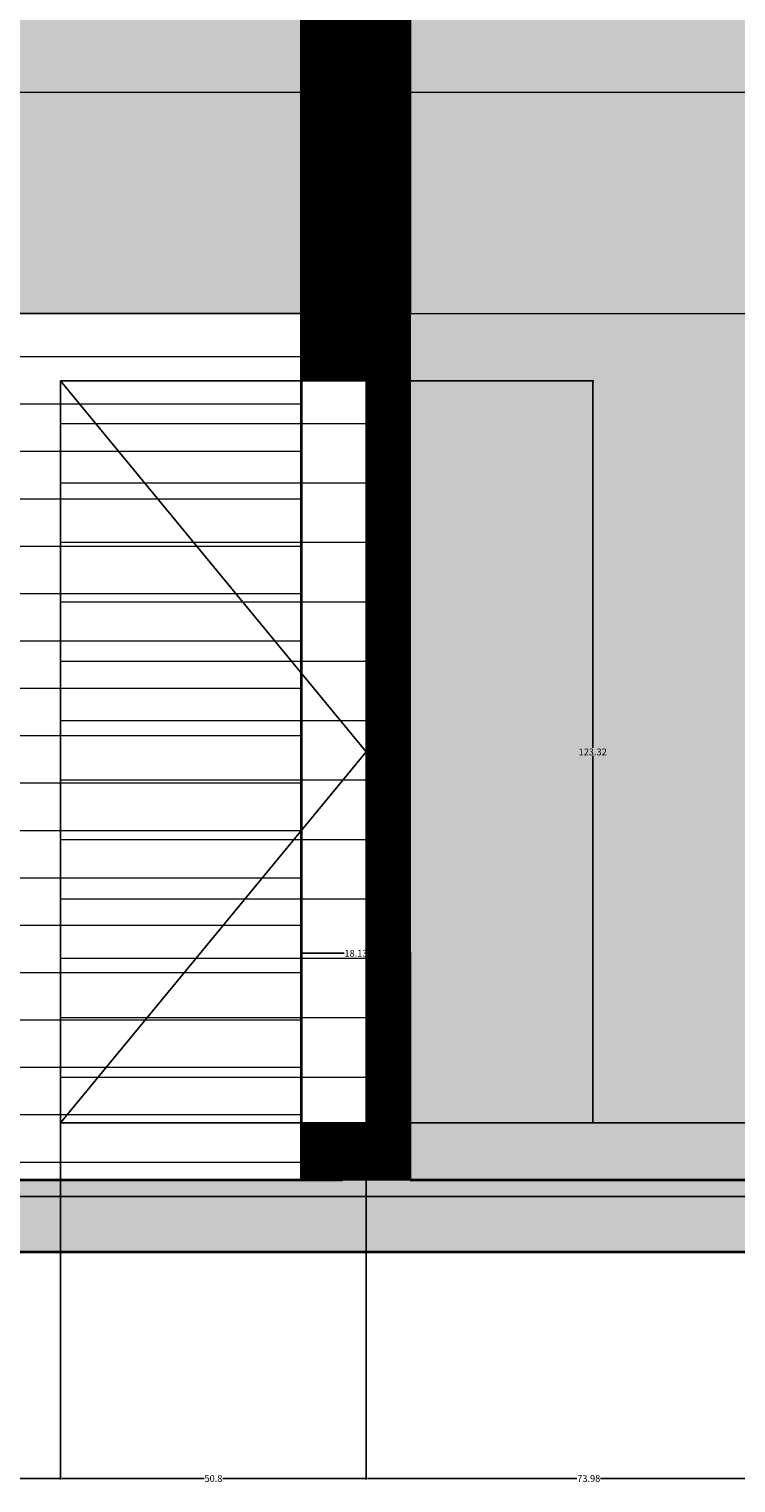
# Model space of a CAD drawing. Units: inches. Extents: x 8 to 634, y 41 to 867.
# Tile 7 of 21: x 297 to 415, y 41 to 283. Entities that reach past the tile are written whole.
import ezdxf

# ---------------------------------------------------------------- set-up
doc = ezdxf.new("R2010")
doc.units = ezdxf.units.IN
doc.header["$MEASUREMENT"] = 0
for name, color, linetype, lineweight in [('A-ANNO-DIMS', 2, 'Continuous', 18), ('A-DOOR', 3, 'Continuous', 25), ('A-ELEV-PATT', 252, 'Continuous', 9), ('A-FLOR', 7, 'Continuous', 35), ('A-FLOR-PATT', 8, 'Continuous', 9), ('A-WALL', 7, 'Continuous', 35), ('A-WALL-PANL', 7, 'Continuous', 18), ('A-WALL-PATT', 8, 'Continuous', 9)]:
    doc.layers.add(name, color=color, linetype=linetype, lineweight=lineweight)
doc.layers.add('A-GLAZ-PATT', color=251, linetype='Continuous', lineweight=9, true_color=0x636466)
doc.styles.get("Standard").update_dxf_attribs({"font": 'arial.ttf'})
doc.dimstyles.get("Standard").update_dxf_attribs({"dimtxt": 1.125, "dimasz": 0.18, "dimexe": 0.18, "dimexo": 0.0625, "dimgap": 0.09, "dimtad": 0, "dimtih": 1, "dimtoh": 1, "dimdec": 4, "dimzin": 0, "dimdsep": 46, "dimlunit": 4, "dimtxsty": 'Standard', "dimcen": 0.09, "dimadec": 0, "dimazin": 0, "dimtfac": 1, "dimtdec": 4, "dimtofl": 0, "dimtmove": 0, "dimatfit": 3, "dimfxl": 1, "dimtolj": 1, "dimtzin": 0, "dimarcsym": 0})

# ---------------------------------------------------------------- blocks, each defined once
blk = doc.blocks.new('*D30')
at = {"layer": 'A-ANNO-DIMS', "color": 0, "lineweight": -2, "transparency": 16777216}
for p, q in [((302.65, 100.94), (302.65, 41.73)), ((269, 88.73), (269, 41.73)), ((269.18, 41.91), (283.4, 41.91)), ((302.47, 41.91), (288.25, 41.91))]:
    blk.add_line(p, q, dxfattribs=at)
at = {"layer": 'A-ANNO-DIMS', "color": 0, "transparency": 16777216}
for points in [[(269.18, 41.94), (269.18, 41.88), (269, 41.91)], [(302.47, 41.94), (302.47, 41.88), (302.65, 41.91)]]:
    blk.add_solid(points, dxfattribs=at)
at = {"layer": 'Defpoints', "color": 0, "transparency": 16777216}
for p in [(302.65, 101), (269, 88.79), (302.65, 41.91)]:
    blk.add_point(p, dxfattribs=at)
at = {"layer": 'A-ANNO-DIMS', "color": 0, "transparency": 16777216, "insert": (285.83, 41.91), "char_height": 1.125, "attachment_point": 5}
blk.add_mtext('\\A1;33.654', dxfattribs=at)
blk = doc.blocks.new('*D31')
at = {"layer": 'A-ANNO-DIMS', "color": 0, "lineweight": -2, "transparency": 16777216}
for p, q in [((302.65, 100.94), (302.65, 41.73)), ((353.46, 100.94), (353.46, 41.73)), ((302.83, 41.91), (326.5, 41.91)), ((353.28, 41.91), (329.61, 41.91))]:
    blk.add_line(p, q, dxfattribs=at)
at = {"layer": 'A-ANNO-DIMS', "color": 0, "transparency": 16777216}
for points in [[(302.83, 41.94), (302.83, 41.88), (302.65, 41.91)], [(353.28, 41.94), (353.28, 41.88), (353.46, 41.91)]]:
    blk.add_solid(points, dxfattribs=at)
at = {"layer": 'Defpoints', "color": 0, "transparency": 16777216}
for p in [(302.65, 101), (353.46, 101), (353.46, 41.91)]:
    blk.add_point(p, dxfattribs=at)
at = {"layer": 'A-ANNO-DIMS', "color": 0, "transparency": 16777216, "insert": (328.05, 41.91), "char_height": 1.125, "attachment_point": 5}
blk.add_mtext('\\A1;50.8', dxfattribs=at)
blk = doc.blocks.new('*D32')
at = {"layer": 'A-ANNO-DIMS', "color": 0, "lineweight": -2, "transparency": 16777216}
for p, q in [((427.44, 124.17), (427.44, 41.73)), ((353.46, 100.94), (353.46, 41.73)), ((353.64, 41.91), (388.46, 41.91)), ((427.26, 41.91), (392.43, 41.91))]:
    blk.add_line(p, q, dxfattribs=at)
at = {"layer": 'A-ANNO-DIMS', "color": 0, "transparency": 16777216}
for points in [[(353.64, 41.94), (353.64, 41.88), (353.46, 41.91)], [(427.26, 41.94), (427.26, 41.88), (427.44, 41.91)]]:
    blk.add_solid(points, dxfattribs=at)
at = {"layer": 'Defpoints', "color": 0, "transparency": 16777216}
for p in [(427.44, 124.23), (353.46, 101), (427.44, 41.91)]:
    blk.add_point(p, dxfattribs=at)
at = {"layer": 'A-ANNO-DIMS', "color": 0, "transparency": 16777216, "insert": (390.45, 41.91), "char_height": 1.125, "attachment_point": 5}
blk.add_mtext('\\A1;73.98', dxfattribs=at)
blk = doc.blocks.new('*D35')
at = {"layer": 'A-ANNO-DIMS', "color": 0, "lineweight": -2, "transparency": 16777216}
for p, q in [((353.52, 224.33), (391.29, 224.33)), ((391.11, 224.15), (391.11, 163.33)), ((391.11, 101.18), (391.11, 162)), ((353.52, 101), (391.29, 101))]:
    blk.add_line(p, q, dxfattribs=at)
at = {"layer": 'A-ANNO-DIMS', "color": 0, "transparency": 16777216}
for points in [[(391.08, 224.15), (391.14, 224.15), (391.11, 224.33)], [(391.08, 101.18), (391.14, 101.18), (391.11, 101)]]:
    blk.add_solid(points, dxfattribs=at)
at = {"layer": 'Defpoints', "color": 0, "transparency": 16777216}
for p in [(353.46, 224.33), (353.46, 101), (391.11, 101)]:
    blk.add_point(p, dxfattribs=at)
at = {"layer": 'A-ANNO-DIMS', "color": 0, "transparency": 16777216, "insert": (391.11, 162.66), "char_height": 1.125, "attachment_point": 5}
blk.add_mtext('\\A1;123.32', dxfattribs=at)
blk = doc.blocks.new('*D36')
at = {"layer": 'A-ANNO-DIMS', "color": 0, "lineweight": -2, "transparency": 16777216}
for p, q in [((269.06, 88.79), (632.18, 88.79)), ((632, 88.61), (632, 84.84)), ((632, 79.74), (632, 83.51)), ((594.41, 79.56), (632.18, 79.56))]:
    blk.add_line(p, q, dxfattribs=at)
at = {"layer": 'A-ANNO-DIMS', "color": 0, "transparency": 16777216}
for points in [[(631.97, 88.61), (632.03, 88.61), (632, 88.79)], [(631.97, 79.74), (632.03, 79.74), (632, 79.56)]]:
    blk.add_solid(points, dxfattribs=at)
at = {"layer": 'Defpoints', "color": 0, "transparency": 16777216}
for p in [(269, 88.79), (632, 88.79), (594.35, 79.56)]:
    blk.add_point(p, dxfattribs=at)
at = {"layer": 'A-ANNO-DIMS', "color": 0, "transparency": 16777216, "insert": (632, 84.17), "char_height": 1.125, "attachment_point": 5}
blk.add_mtext('\\A1;9.236', dxfattribs=at)
blk = doc.blocks.new('*D37')
at = {"layer": 'A-ANNO-DIMS', "color": 0, "lineweight": -2, "transparency": 16777216}
for p, q in [((353.52, 101), (632.18, 101)), ((632, 100.82), (632, 95.55)), ((632, 88.97), (632, 94.24)), ((269.06, 88.79), (632.18, 88.79))]:
    blk.add_line(p, q, dxfattribs=at)
at = {"layer": 'A-ANNO-DIMS', "color": 0, "transparency": 16777216}
for points in [[(631.97, 100.82), (632.03, 100.82), (632, 101)], [(631.97, 88.97), (632.03, 88.97), (632, 88.79)]]:
    blk.add_solid(points, dxfattribs=at)
at = {"layer": 'Defpoints', "color": 0, "transparency": 16777216}
for p in [(353.46, 101), (632, 101), (269, 88.79)]:
    blk.add_point(p, dxfattribs=at)
at = {"layer": 'A-ANNO-DIMS', "color": 0, "transparency": 16777216, "insert": (632, 94.9), "char_height": 1.125, "attachment_point": 5}
blk.add_mtext('\\A1;12.21', dxfattribs=at)
blk = doc.blocks.new('*D38')
at = {"layer": 'A-ANNO-DIMS', "color": 0, "lineweight": -2, "transparency": 16777216}
for p, q in [((427.5, 124.23), (632.18, 124.23)), ((632, 124.05), (632, 113.28)), ((632, 101.18), (632, 111.95)), ((353.52, 101), (632.18, 101))]:
    blk.add_line(p, q, dxfattribs=at)
at = {"layer": 'A-ANNO-DIMS', "color": 0, "transparency": 16777216}
for points in [[(631.97, 124.05), (632.03, 124.05), (632, 124.23)], [(631.97, 101.18), (632.03, 101.18), (632, 101)]]:
    blk.add_solid(points, dxfattribs=at)
at = {"layer": 'Defpoints', "color": 0, "transparency": 16777216}
for p in [(427.44, 124.23), (632, 124.23), (353.46, 101)]:
    blk.add_point(p, dxfattribs=at)
at = {"layer": 'A-ANNO-DIMS', "color": 0, "transparency": 16777216, "insert": (632, 112.62), "char_height": 1.125, "attachment_point": 5}
blk.add_mtext('\\A1;23.233', dxfattribs=at)
blk = doc.blocks.new('*D64')
at = {"layer": 'A-ANNO-DIMS', "color": 0, "lineweight": -2, "transparency": 16777216}
for p, q in [((342.65, 91.62), (342.68, 129.39)), ((342.86, 129.21), (349.81, 129.2)), ((360.63, 129.19), (353.68, 129.2)), ((360.79, 91.6), (360.81, 129.37))]:
    blk.add_line(p, q, dxfattribs=at)
at = {"layer": 'A-ANNO-DIMS', "color": 0, "transparency": 16777216}
for points in [[(342.86, 129.24), (342.86, 129.18), (342.68, 129.21)], [(360.63, 129.22), (360.63, 129.16), (360.81, 129.19)]]:
    blk.add_solid(points, dxfattribs=at)
at = {"layer": 'Defpoints', "color": 0, "transparency": 16777216}
for p in [(360.81, 129.19), (342.65, 91.56), (360.79, 91.54)]:
    blk.add_point(p, dxfattribs=at)
at = {"layer": 'A-ANNO-DIMS', "color": 0, "transparency": 16777216, "insert": (351.75, 129.2), "char_height": 1.125, "attachment_point": 5}
blk.add_mtext('\\A1;18.13', dxfattribs=at)

msp = doc.modelspace()

# ---------------------------------------------------------------- hatches: boundary and pattern name
at = {"layer": 'A-ELEV-PATT', "transparency": 33554544}
h = msp.add_hatch(dxfattribs=at)
h.set_pattern_fill('ANSI31', color=256)
h.paths.add_polyline_path([(360.785, 697.6655), (342.6544, 682.1444), (342.6544, 569.1705), (360.785, 569.1705)])
h.paths.add_polyline_path([(360.785, 523.5555), (360.785, 569.1705), (342.6544, 569.1705), (342.6544, 449.7533), (360.785, 449.7533)])
h.paths.add_polyline_path([(360.785, 449.7533), (342.6544, 449.7533), (342.6544, 391.7598), (360.785, 391.7598)])
h.paths.add_polyline_path([(360.785, 391.7598), (342.6544, 391.7598), (342.6544, 272.3426), (360.785, 272.3426)])
h.paths.add_polyline_path([(360.785, 272.3426), (342.6544, 272.3426), (342.6544, 235.5555), (360.785, 235.5555)])
h.paths.add_polyline_path([(360.785, 235.5555), (342.6544, 235.5555), (342.6544, 224.3257), (353.4573, 224.3257), (353.4573, 101.0012), (342.6544, 101.0012), (342.6544, 91.5417), (360.785, 91.5417)])
at = {"layer": 'A-FLOR-PATT', "transparency": 33554687}
h = msp.add_hatch(dxfattribs=at)
h.set_pattern_fill('AR-CONC', color=256, scale=0.76, angle=135)
h.set_pattern_definition([(185, (0, 0), (-3.517334, 4.191795), [0.57, -6.27]), (130, (0, 0), (-3.29664, -4.78794), [0.456, -5.016]), (235.4514, (-0.293, 0.3493), (-6.81397, -0.596145), [0.484425, -5.32868]), (181.1842, (-1.075, -1.075), (-4.845865, 6.62487), [0.855, -9.405]), (231.6356, (-1.479, -0.523), (-10.25781, -0.21204), [0.72664, -7.99302]), (126.1842, (-1.075, -1.075), (-10.25781, -0.21204), [0.684, -7.524]), (156, (-1.3435, -0.2687), (-1.044107, 5.371464), [0.57, -6.27]), (101, (-1.3435, -0.2687), (-5.204544, -2.589385), [0.456, -5.016]), (206.4514, (-1.4305, 0.179), (-6.24865, 2.78208), [0.484425, -5.32868]), (172.5, (0, 0), (-1.8543226, -1.723628), [0, -4.9552, 0, -5.092, 0, -5.035]), (142.5, (0, 0), (-3.533312, -0.705834), [0, -2.9032, 0, -4.8412, 0, -1.919]), (102.5, (1.1984, -1.1984), (-2.747558, 2.989978), [0, -1.9, 0, -5.928, 0, -7.866]), (92.5, (1.7358, -1.7358), (-3.672015, 2.596084), [0, -2.47, 0, -3.9368, 0, -5.586])])
h.paths.add_polyline_path([(594.3501, 91.5417), (360.785, 91.5417), (295.0049, 91.5417), (268.998, 91.5432), (268.998, 88.7912), (63.5448, 88.7912), (63.5448, 91.5555), (47.3401, 91.5555), (47.3401, 79.5555), (349.489, 79.5555), (594.3501, 79.5555)])
at = {"layer": 'A-GLAZ-PATT', "transparency": 33554687}
h = msp.add_hatch(dxfattribs=at)
h.set_pattern_fill('ANSI31', color=256, scale=79, angle=135)
h.paths.add_polyline_path([(355.7466, 740.5561), (322.56, 740.5561), (322.56, 697.6655), (355.7466, 697.6655)])
h.paths.add_polyline_path([(439.201, 740.5561), (370.3877, 740.5561), (370.3877, 697.6655), (418.2881, 697.6655), (418.2881, 691.978), (439.201, 691.978)])
h.paths.add_polyline_path([(498.2535, 740.5561), (449.4498, 740.5561), (449.4498, 691.978), (498.2535, 691.978)])
h.paths.add_polyline_path([(536.3204, 740.5561), (508.5023, 740.5561), (508.5023, 691.978), (536.3204, 691.978)])
h.paths.add_polyline_path([(439.201, 690.978), (418.2881, 690.978), (418.2881, 682.0586), (439.201, 682.0586)])
h.paths.add_polyline_path([(439.201, 681.0586), (418.2881, 681.0586), (418.2881, 673.2414), (439.201, 673.2414)])
h.paths.add_polyline_path([(439.201, 672.2414), (418.2881, 672.2414), (418.2881, 662.4168), (439.201, 662.4168)])
h.paths.add_polyline_path([(439.201, 661.4168), (418.2881, 661.4168), (418.2881, 651.537), (439.201, 651.537)])
h.paths.add_polyline_path([(439.201, 650.537), (418.2881, 650.537), (418.2881, 640.7358), (439.201, 640.7358)])
h.paths.add_polyline_path([(439.201, 639.7358), (418.2881, 639.7358), (418.2881, 630.9186), (439.201, 630.9186)])
h.paths.add_polyline_path([(439.201, 629.9186), (418.2881, 629.9186), (418.2881, 619.6298), (439.201, 619.6298)])
h.paths.add_polyline_path([(477.6441, 629.9186), (449.4498, 629.9186), (449.4498, 619.6298), (477.6441, 619.6298)])
h.paths.add_polyline_path([(477.6441, 639.7358), (449.4498, 639.7358), (449.4498, 630.9186), (477.6441, 630.9186)])
h.paths.add_polyline_path([(477.6441, 650.537), (449.4498, 650.537), (449.4498, 640.7358), (477.6441, 640.7358)])
h.paths.add_polyline_path([(477.6441, 661.4168), (449.4498, 661.4168), (449.4498, 651.537), (477.6441, 651.537)])
h.paths.add_polyline_path([(477.6441, 672.2414), (449.4498, 672.2414), (449.4498, 662.4168), (477.6441, 662.4168)])
h.paths.add_polyline_path([(477.6441, 681.0586), (449.4498, 681.0586), (449.4498, 673.2414), (477.6441, 673.2414)])
h.paths.add_polyline_path([(477.6441, 690.978), (449.4498, 690.978), (449.4498, 682.0586), (477.6441, 682.0586)])
h.paths.add_polyline_path([(498.2535, 690.978), (478.6441, 690.978), (478.6441, 682.0586), (498.2535, 682.0586)])
h.paths.add_polyline_path([(498.2535, 681.0586), (478.6441, 681.0586), (478.6441, 673.2414), (498.2535, 673.2414)])
h.paths.add_polyline_path([(498.2535, 672.2414), (478.6441, 672.2414), (478.6441, 662.4168), (498.2535, 662.4168)])
h.paths.add_polyline_path([(498.2535, 661.4168), (478.6441, 661.4168), (478.6441, 651.537), (498.2535, 651.537)])
h.paths.add_polyline_path([(498.2535, 650.537), (478.6441, 650.537), (478.6441, 640.7358), (498.2535, 640.7358)])
h.paths.add_polyline_path([(498.2535, 639.7358), (478.6441, 639.7358), (478.6441, 630.9186), (498.2535, 630.9186)])
h.paths.add_polyline_path([(498.2535, 629.9186), (478.6441, 629.9186), (478.6441, 619.6298), (498.2535, 619.6298)])
h.paths.add_polyline_path([(536.3204, 629.9186), (508.5023, 629.9186), (508.5023, 619.6298), (536.3204, 619.6298)])
h.paths.add_polyline_path([(536.3204, 639.7358), (508.5023, 639.7358), (508.5023, 630.9186), (536.3204, 630.9186)])
h.paths.add_polyline_path([(536.3204, 650.537), (508.5023, 650.537), (508.5023, 640.7358), (536.3204, 640.7358)])
h.paths.add_polyline_path([(536.3204, 661.4168), (508.5023, 661.4168), (508.5023, 651.537), (536.3204, 651.537)])
h.paths.add_polyline_path([(536.3204, 672.2414), (508.5023, 672.2414), (508.5023, 662.4168), (536.3204, 662.4168)])
h.paths.add_polyline_path([(536.3204, 681.0586), (508.5023, 681.0586), (508.5023, 673.2414), (536.3204, 673.2414)])
h.paths.add_polyline_path([(536.3204, 690.978), (508.5023, 690.978), (508.5023, 682.0586), (536.3204, 682.0586)])
h.paths.add_polyline_path([(342.6544, 175.7749), (302.6522, 224.3257), (302.6522, 101.0012), (342.6544, 149.552)])
h.paths.add_polyline_path([(342.6544, 224.3257), (302.6522, 224.3257), (342.6544, 175.7749)])
h.paths.add_polyline_path([(342.6544, 149.552), (302.6522, 101.0012), (342.6544, 101.0012)])
h.paths.add_polyline_path([(353.4573, 162.6634), (342.6544, 149.552), (342.6544, 101.0012), (353.4573, 101.0012)])
h.paths.add_polyline_path([(353.4573, 224.3257), (342.6544, 224.3257), (342.6544, 101.0012), (353.4573, 101.0012)])
h.paths.add_polyline_path([(342.6544, 175.7749), (342.6544, 149.552), (353.4573, 162.6634)], flags=17)
h = msp.add_hatch(dxfattribs=at)
h.set_pattern_fill('ANSI31', color=256, scale=79, angle=135)
h.paths.add_polyline_path([(353.4573, 162.6634), (342.6544, 149.552), (342.6544, 101.0012), (353.4573, 101.0012)])
h.paths.add_polyline_path([(342.6544, 175.7749), (342.6544, 149.552), (353.4573, 162.6634)])
at = {"layer": 'A-WALL-PATT', "transparency": 33554687}
h = msp.add_hatch(dxfattribs=at)
h.set_pattern_fill('AR-CONC', color=256, scale=3.2)
h.paths.add_polyline_path([(119.7065, 697.6655), (47.3401, 697.6655), (47.3401, 569.1705), (119.7065, 569.1705)])
h.paths.add_polyline_path([(202.1558, 697.6655), (119.7065, 697.6655), (119.7065, 569.1705), (202.1558, 569.1705)])
h.paths.add_polyline_path([(284.6051, 697.6655), (202.1558, 697.6655), (202.1558, 569.1705), (284.6051, 569.1705)])
h.paths.add_polyline_path([(119.7065, 569.1705), (47.3401, 569.1705), (47.3401, 523.5555), (47.3401, 449.7533), (119.7065, 449.7533)])
h.paths.add_polyline_path([(342.6544, 682.1444), (360.785, 697.6655), (284.6051, 697.6655), (284.6051, 569.1705), (342.6544, 569.1705)])
h.paths.add_polyline_path([(342.6544, 569.1705), (284.6051, 569.1705), (284.6051, 449.7533), (342.6544, 449.7533)])
h.paths.add_polyline_path([(418.2881, 691.978), (418.2881, 697.6655), (360.785, 697.6655), (360.785, 569.1705), (418.2881, 569.1705)])
h.paths.add_polyline_path([(418.2881, 569.1705), (360.785, 569.1705), (360.785, 523.5555), (360.785, 449.7533), (418.2881, 449.7533)])
h.paths.add_polyline_path([(594.3501, 697.6655), (539.0002, 697.6655), (539.0002, 691.978), (539.0002, 569.1705), (594.3501, 569.1705)])
h.paths.add_polyline_path([(594.3501, 523.5555), (594.3501, 569.1705), (539.0002, 569.1705), (539.0002, 451.6305), (594.3501, 451.6305)])
h.paths.add_polyline_path([(594.3501, 451.6305), (539.0002, 451.6305), (539.0002, 391.7598), (594.3501, 391.7598)])
h.paths.add_polyline_path([(594.3501, 391.7598), (539.0002, 391.7598), (539.0002, 276.166), (594.3501, 276.166)])
h.paths.add_polyline_path([(418.2881, 449.7533), (360.785, 449.7533), (360.785, 391.7598), (418.2881, 391.7598)])
h.paths.add_polyline_path([(342.6544, 449.7533), (284.6051, 449.7533), (284.6051, 391.7598), (342.6544, 391.7598)])
h.paths.add_polyline_path([(342.6544, 391.7598), (284.6051, 391.7598), (284.6051, 272.3426), (342.6544, 272.3426)])
h.paths.add_polyline_path([(418.2881, 391.7598), (360.785, 391.7598), (360.785, 272.3426), (418.2881, 272.3426)])
h.paths.add_polyline_path([(418.2881, 272.3426), (360.785, 272.3426), (360.785, 235.5555), (418.2881, 235.5555)])
h.paths.add_polyline_path([(342.6544, 272.3426), (284.6051, 272.3426), (284.6051, 235.5555), (295.0049, 235.5555), (342.6544, 235.5555)])
h.paths.add_polyline_path([(594.3501, 276.166), (539.0002, 276.166), (539.0002, 228.4951), (594.3501, 228.4951)])
h.paths.add_polyline_path([(594.3501, 228.4951), (539.0002, 228.4951), (539.0002, 91.5417), (594.3501, 91.5417)])
h.paths.add_polyline_path([(418.2881, 235.5555), (360.785, 235.5555), (360.785, 91.5417), (418.2881, 91.5417)])
h.paths.add_polyline_path([(284.6051, 272.3426), (119.7065, 272.3426), (119.7065, 235.5555), (284.6051, 235.5555)])
h.paths.add_polyline_path([(119.7065, 272.3426), (47.3401, 272.3426), (47.3401, 235.5555), (47.3401, 91.5555), (63.5448, 91.5555), (63.5448, 227.8036), (268.998, 227.8036), (268.998, 91.5555), (295.0049, 91.5555), (295.0049, 222.583), (271.9787, 222.583), (271.9787, 229.0481), (62.4019, 229.0481), (62.4019, 222.583), (61.1827, 222.583), (61.1827, 235.5555), (119.7065, 235.5555)])
h.paths.add_polyline_path([(119.7065, 391.7598), (47.3401, 391.7598), (47.3401, 379.5555), (47.3401, 272.3426), (119.7065, 272.3426)])
h.paths.add_polyline_path([(119.7065, 449.7533), (47.3401, 449.7533), (47.3401, 391.7598), (119.7065, 391.7598)])
h.paths.add_polyline_path([(202.1558, 449.7533), (119.7065, 449.7533), (119.7065, 391.7598), (202.1558, 391.7598)])
h.paths.add_polyline_path([(284.6051, 449.7533), (202.1558, 449.7533), (202.1558, 391.7598), (284.6051, 391.7598)])
at = {"layer": 'A-WALL-PATT', "transparency": 33554681}
h = msp.add_hatch(dxfattribs=at)
h.set_pattern_fill('ANSI31', color=256, scale=63, angle=135)
h.paths.add_polyline_path([(284.6051, 391.7598), (119.7065, 391.7598), (119.7065, 272.3426), (284.6051, 272.3426)])
h.paths.add_polyline_path([(193.1116, 284.2398), (131.8771, 284.2398), (131.8771, 380.0085), (193.1116, 380.0085)], flags=16)
h.paths.add_polyline_path([(207.7547, 380.0085), (268.9893, 380.0085), (268.9893, 284.2398), (207.7547, 284.2398)], flags=16)
h.paths.add_polyline_path([(342.6544, 235.5555), (295.0049, 235.5555), (295.0049, 91.5417), (342.6544, 91.5417)])

# ---------------------------------------------------------------- linework, layer by layer
at = {"layer": 'A-DOOR'}
for p, q in [((302.6522, 224.3257), (353.4573, 162.6634)), ((353.4573, 162.6634), (302.6522, 101.0012))]:
    msp.add_line(p, q, dxfattribs=at)
for points in [[(295.0049, 235.5555), (360.785, 235.5555), (360.785, 91.5417), (295.0049, 91.5417)], [(302.6522, 224.3257), (353.4573, 224.3257), (353.4573, 101.0012), (302.6522, 101.0012)]]:
    msp.add_lwpolyline(points, close=True, dxfattribs=at)
at = {"layer": 'A-FLOR'}
for p, q in [((47.3401, 91.5555), (349.489, 91.5555)), ((360.785, 91.5417), (594.3501, 91.5417)), ((47.3401, 79.5555), (349.489, 79.5555)), ((349.489, 79.5555), (594.3501, 79.5555))]:
    msp.add_line(p, q, dxfattribs=at)
at = {"layer": 'A-WALL'}
for p, q in [((342.6544, 682.1444), (342.6544, 91.5555)), ((360.785, 235.5555), (360.785, 523.5555))]:
    msp.add_line(p, q, dxfattribs=at)
at = {"layer": 'A-WALL-PANL'}
for p, q in [((284.6051, 272.3426), (418.2881, 272.3426)), ((360.785, 235.5555), (418.2881, 235.5555))]:
    msp.add_line(p, q, dxfattribs=at)

# ---------------------------------------------------------------- dimensions: what is measured, and where the dimension line sits
at = {"layer": 'A-ANNO-DIMS'}
for base, p1, p2, angle, override, picture, middle in [((391.1073, 101.0012), (353.4573, 224.3257), (353.4573, 101.0012), 270, {"dimdec": 2, "dimlfac": 1, "dimrnd": 0, "dimzin": 0, "dimdsep": 46, "dimlunit": 2}, '*D35', (391.1073, 162.6634)), ((360.8137, 129.1917), (342.6544, 91.5555), (360.785, 91.5417), 359.956323, {"dimdec": 2, "dimlfac": 1, "dimrnd": 0, "dimzin": 0, "dimdsep": 46, "dimlunit": 2}, '*D64', (351.7484, 129.1986)), ((632.0001, 124.2342), (353.4573, 101.0012), (427.4368, 124.2342), 90, {"dimdec": 3, "dimlfac": 1, "dimrnd": 0, "dimzin": 0, "dimdsep": 46, "dimlunit": 2}, '*D38', (632.0001, 112.6177)), ((632.0001, 101.0012), (268.998, 88.7912), (353.4573, 101.0012), 90, {"dimdec": 2, "dimlfac": 1, "dimrnd": 0, "dimzin": 0, "dimdsep": 46, "dimlunit": 2}, '*D37', (632.0001, 94.8962)), ((632.0001, 88.7912), (594.3501, 79.5555), (268.998, 88.7912), 90, {"dimdec": 3, "dimlfac": 1, "dimrnd": 0, "dimzin": 0, "dimdsep": 46, "dimlunit": 2}, '*D36', (632.0001, 84.1734))]:
    dim = msp.add_linear_dim(base=base, p1=p1, p2=p2, angle=angle, dimstyle='Standard', override=override, dxfattribs=at)
    dim.commit()
    dim.dimension.update_dxf_attribs({"geometry": picture, "text_midpoint": middle})
for base, p1, p2, override, picture, middle in [((427.4368, 41.9055), (353.4573, 101.0012), (427.4368, 124.2342), {"dimdec": 2, "dimlfac": 1, "dimrnd": 0, "dimzin": 0, "dimdsep": 46, "dimlunit": 2}, '*D32', (390.447, 41.9055)), ((302.6522, 41.9055), (268.998, 88.7912), (302.6522, 101.0012), {"dimdec": 3, "dimlfac": 1, "dimrnd": 0, "dimzin": 0, "dimdsep": 46, "dimlunit": 2}, '*D30', (285.8251, 41.9055)), ((353.4573, 41.9055), (302.6522, 101.0012), (353.4573, 101.0012), {"dimdec": 1, "dimlfac": 1, "dimrnd": 0, "dimzin": 0, "dimdsep": 46, "dimlunit": 2}, '*D31', (328.0547, 41.9055))]:
    dim = msp.add_linear_dim(base=base, p1=p1, p2=p2, dimstyle='Standard', override=override, dxfattribs=at)
    dim.commit()
    dim.dimension.update_dxf_attribs({"geometry": picture, "text_midpoint": middle})

doc.saveas('drawing.dxf')
